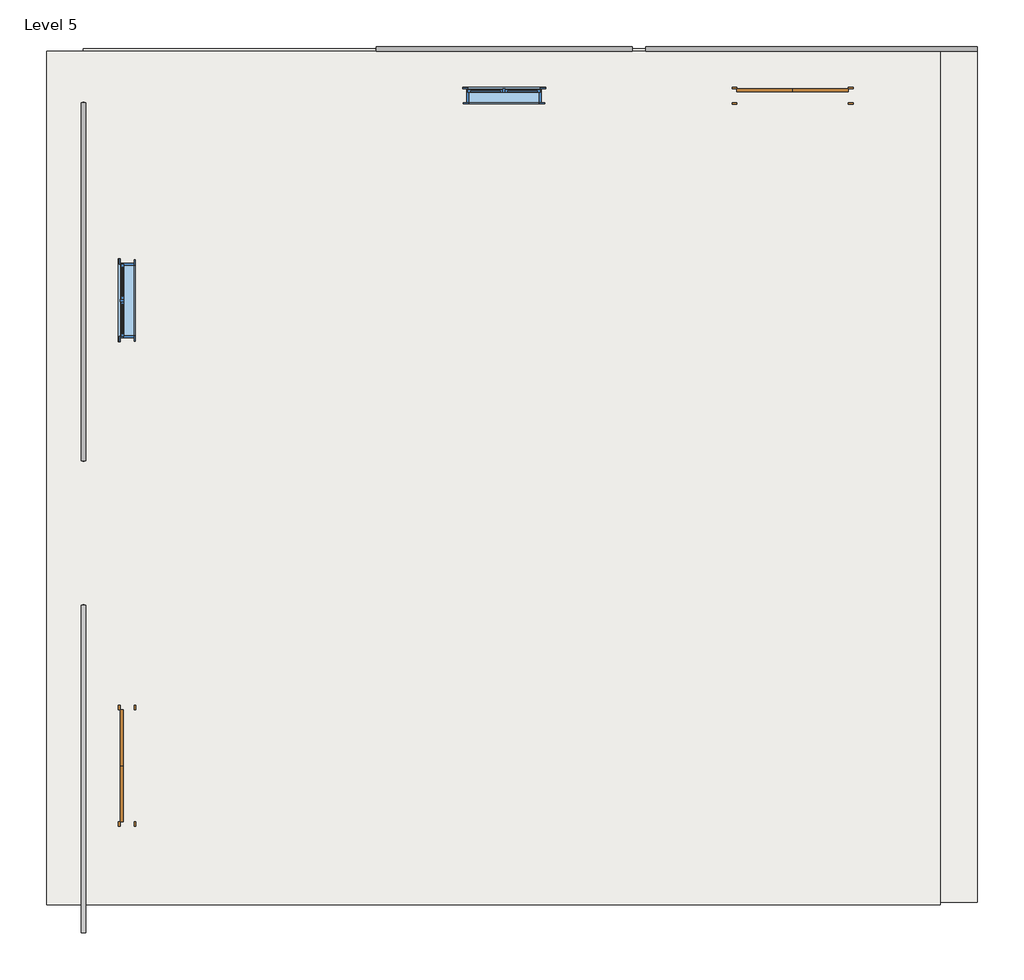
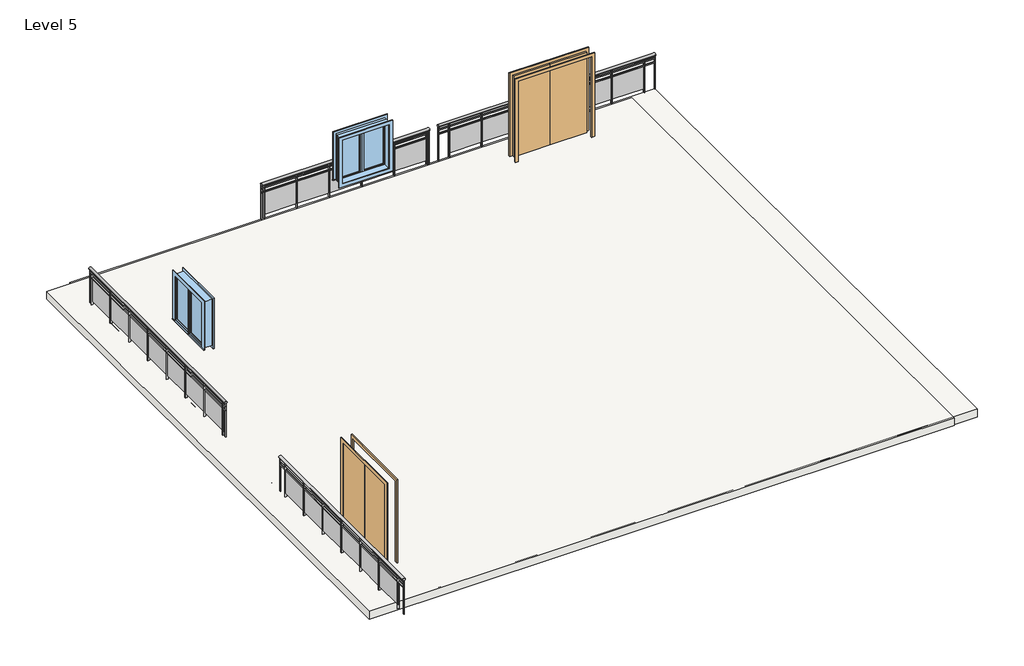
# One storey: 4 railings, 2 doors, 2 slabs, 2 windows.
"""IFC4 building model written with IfcOpenShell, lengths in millimetres."""

from ifc_helpers import new_model, si_unit, point, frame, origin, place, context, project, spatial, polyline, ellipse_curve, trimmed, outline, extrude, transform, mapped, element, save
from ifc_brep_helpers import plane_surface, extruded_surface, advanced_brep
from components import door_640b4634, window_534dcd48

model = new_model("IFC4")

# Units and contexts
model_context = context("Model", 3, world=origin())
ifc_project = project(units=[si_unit("LENGTHUNIT", "METRE", prefix="MILLI")], contexts=[model_context])

# Site, building, storey
site = spatial("IfcSite", under=ifc_project)
building = spatial("IfcBuilding", under=site)
storey = spatial("IfcBuildingStorey", under=building, Name="Level 5", Elevation=12801.6)

# Doors
placement = place(None, origin())
door_shape = door_640b4634(model_context)
element("IfcDoor", 1, ObjectType="Door-Double-Flush_Panel : 72\" x 84\"", at=placement, inside=storey, context=model_context, shape_type="MappedRepresentation", body=[
    mapped(door_shape, transform((-18468.543393, -6784.3397804, 12801.6), x_axis=(0.0, 1.0, 0.0), y_axis=(-1.0, 0.0, 0.0), z_axis=(0.0, 0.0, 1.0))),
])
element("IfcDoor", 2, ObjectType="Door-Double-Flush_Panel : 72\" x 84\"", at=placement, inside=storey, context=model_context, shape_type="MappedRepresentation", body=[
    mapped(door_shape, transform((-7571.943393, 4188.4602196, 12801.6), x_axis=(1.0, 0.0, 0.0), y_axis=(0.0, 1.0, 0.0), z_axis=(0.0, 0.0, 1.0))),
])

# Railings
element("IfcRailing", 3, ObjectType="Glass Panel - Bottom Fill", at=placement, inside=storey, context=model_context, shape_type="SolidModel", body=[
    advanced_brep(
    [(-19220.0296876, -9514.8397804, 13716.0), (-19143.8296876, -9514.8397804, 13716.0), (-19220.0296876, -4155.4397804, 13716.0), (-19143.8296876, -4155.4397804, 13716.0)],
    [
        (0, 1, ellipse_curve(frame((-19181.9296876, -9514.8397804, 13716.0), z_axis=(0.0, -1.0, 0.0), x_axis=(1.0, 0.0, 0.0)), 38.1, 28.575)),
        (1, 0, ellipse_curve(frame((-19181.9296876, -9514.8397804, 13716.0), z_axis=(0.0, -1.0, 0.0), x_axis=(1.0, 0.0, 0.0)), 38.1, 28.575)),
        (2, 3, ellipse_curve(frame((-19181.9296876, -4155.4397804, 13716.0), z_axis=(0.0, 1.0, 0.0), x_axis=(1.0, 0.0, 0.0)), 38.1, 28.575)),
        (3, 2, ellipse_curve(frame((-19181.9296876, -4155.4397804, 13716.0), z_axis=(0.0, 1.0, 0.0), x_axis=(1.0, 0.0, 0.0)), 38.1, 28.575)),
        (0, 2),
        (3, 1),
    ],
    [
        plane_surface(frame((-19181.9296876, -9514.8397804, 13716.0), z_axis=(0.0, -1.0, 0.0), x_axis=(0.0, 0.0, 1.0))),
        plane_surface(frame((-19181.9296876, -4155.4397804, 13716.0), z_axis=(0.0, 1.0, 0.0), x_axis=(0.0, 0.0, 1.0))),
        extruded_surface(trimmed(ellipse_curve(frame((-19181.9296876, -4155.4397804, 13716.0), z_axis=(0.0, -1.0, 0.0), x_axis=(1.0, 0.0, 0.0)), 38.1, 28.575), [point((-19220.0296876, -4155.4397804, 13716.0))], [point((-19143.8296876, -4155.4397804, 13716.0))], True, "CARTESIAN"), (0.0, -5359.4, 0.0), 5359.4),
        extruded_surface(trimmed(ellipse_curve(frame((-19181.9296876, -4155.4397804, 13716.0), z_axis=(0.0, -1.0, 0.0), x_axis=(1.0, 0.0, 0.0)), 38.1, 28.575), [point((-19143.8296876, -4155.4397804, 13716.0))], [point((-19220.0296876, -4155.4397804, 13716.0))], True, "CARTESIAN"), (0.0, -5359.4, 0.0), 5359.4),
    ],
    [
        (0, [[1, 2]]),
        (1, [[3, 4]]),
        (2, [[-1, 5, -4, 6]]),
        (3, [[-2, -6, -3, -5]]),
    ],
),
    extrude(outline(polyline([(-19169.2296876, -9514.8397804), (-19194.6296876, -9514.8397804), (-19194.6296876, -4155.4397804), (-19169.2296876, -4155.4397804), (-19169.2296876, -9514.8397804)])), frame((0.0, 0.0, 13601.7), z_axis=(0.0, 0.0, 1.0), x_axis=(1.0, 0.0, 0.0)), (0.0, 0.0, 1.0), 25.4),
    extrude(outline(polyline([(-19169.2296876, -9514.8397804), (-19194.6296876, -9514.8397804), (-19194.6296876, -4155.4397804), (-19169.2296876, -4155.4397804), (-19169.2296876, -9514.8397804)])), frame((0.0, 0.0, 13500.1), z_axis=(0.0, 0.0, 1.0), x_axis=(1.0, 0.0, 0.0)), (0.0, 0.0, 1.0), 25.4),
    extrude(outline(polyline([(-19156.5296876, -4403.0897804), (-19207.3296876, -4403.0897804), (-19207.3296876, -4390.3897804), (-19156.5296876, -4390.3897804), (-19156.5296876, -4403.0897804)])), frame((0.0, 0.0, 12801.6), z_axis=(0.0, 0.0, 1.0), x_axis=(1.0, 0.0, 0.0)), (0.0, 0.0, 1.0), 885.6788223),
    extrude(outline(polyline([(-19188.4648446, -5209.5397804), (-19188.4648446, -4396.7397804), (-19182.1148446, -4396.7397804), (-19182.1148446, -5209.5397804), (-19188.4648446, -5209.5397804)])), frame((0.0, 0.0, 12903.2), z_axis=(0.0, 0.0, 1.0), x_axis=(1.0, 0.0, 0.0)), (0.0, 0.0, 1.0), 596.9),
    extrude(outline(polyline([(-19156.5296876, -5215.8897804), (-19207.3296876, -5215.8897804), (-19207.3296876, -5203.1897804), (-19156.5296876, -5203.1897804), (-19156.5296876, -5215.8897804)])), frame((0.0, 0.0, 12801.6), z_axis=(0.0, 0.0, 1.0), x_axis=(1.0, 0.0, 0.0)), (0.0, 0.0, 1.0), 885.6788223),
    extrude(outline(polyline([(-19188.4648446, -6022.3397804), (-19188.4648446, -5209.5397804), (-19182.1148446, -5209.5397804), (-19182.1148446, -6022.3397804), (-19188.4648446, -6022.3397804)])), frame((0.0, 0.0, 12903.2), z_axis=(0.0, 0.0, 1.0), x_axis=(1.0, 0.0, 0.0)), (0.0, 0.0, 1.0), 596.9),
    extrude(outline(polyline([(-19156.5296876, -6028.6897804), (-19207.3296876, -6028.6897804), (-19207.3296876, -6015.9897804), (-19156.5296876, -6015.9897804), (-19156.5296876, -6028.6897804)])), frame((0.0, 0.0, 12801.6), z_axis=(0.0, 0.0, 1.0), x_axis=(1.0, 0.0, 0.0)), (0.0, 0.0, 1.0), 885.6788223),
    extrude(outline(polyline([(-19188.4648446, -6835.1397804), (-19188.4648446, -6022.3397804), (-19182.1148446, -6022.3397804), (-19182.1148446, -6835.1397804), (-19188.4648446, -6835.1397804)])), frame((0.0, 0.0, 12903.2), z_axis=(0.0, 0.0, 1.0), x_axis=(1.0, 0.0, 0.0)), (0.0, 0.0, 1.0), 596.9),
    extrude(outline(polyline([(-19156.5296876, -6841.4897804), (-19207.3296876, -6841.4897804), (-19207.3296876, -6828.7897804), (-19156.5296876, -6828.7897804), (-19156.5296876, -6841.4897804)])), frame((0.0, 0.0, 12801.6), z_axis=(0.0, 0.0, 1.0), x_axis=(1.0, 0.0, 0.0)), (0.0, 0.0, 1.0), 885.6788223),
    extrude(outline(polyline([(-19188.4648446, -7647.9397804), (-19188.4648446, -6835.1397804), (-19182.1148446, -6835.1397804), (-19182.1148446, -7647.9397804), (-19188.4648446, -7647.9397804)])), frame((0.0, 0.0, 12903.2), z_axis=(0.0, 0.0, 1.0), x_axis=(1.0, 0.0, 0.0)), (0.0, 0.0, 1.0), 596.9),
    extrude(outline(polyline([(-19156.5296876, -7654.2897804), (-19207.3296876, -7654.2897804), (-19207.3296876, -7641.5897804), (-19156.5296876, -7641.5897804), (-19156.5296876, -7654.2897804)])), frame((0.0, 0.0, 12801.6), z_axis=(0.0, 0.0, 1.0), x_axis=(1.0, 0.0, 0.0)), (0.0, 0.0, 1.0), 885.6788223),
    extrude(outline(polyline([(-19188.4648446, -8460.7397804), (-19188.4648446, -7647.9397804), (-19182.1148446, -7647.9397804), (-19182.1148446, -8460.7397804), (-19188.4648446, -8460.7397804)])), frame((0.0, 0.0, 12903.2), z_axis=(0.0, 0.0, 1.0), x_axis=(1.0, 0.0, 0.0)), (0.0, 0.0, 1.0), 596.9),
    extrude(outline(polyline([(-19156.5296876, -8467.0897804), (-19207.3296876, -8467.0897804), (-19207.3296876, -8454.3897804), (-19156.5296876, -8454.3897804), (-19156.5296876, -8467.0897804)])), frame((0.0, 0.0, 12801.6), z_axis=(0.0, 0.0, 1.0), x_axis=(1.0, 0.0, 0.0)), (0.0, 0.0, 1.0), 885.6788223),
    extrude(outline(polyline([(-19188.4648446, -9273.5397804), (-19188.4648446, -8460.7397804), (-19182.1148446, -8460.7397804), (-19182.1148446, -9273.5397804), (-19188.4648446, -9273.5397804)])), frame((0.0, 0.0, 12903.2), z_axis=(0.0, 0.0, 1.0), x_axis=(1.0, 0.0, 0.0)), (0.0, 0.0, 1.0), 596.9),
    extrude(outline(polyline([(-19156.5296876, -9279.8897804), (-19207.3296876, -9279.8897804), (-19207.3296876, -9267.1897804), (-19156.5296876, -9267.1897804), (-19156.5296876, -9279.8897804)])), frame((0.0, 0.0, 12801.6), z_axis=(0.0, 0.0, 1.0), x_axis=(1.0, 0.0, 0.0)), (0.0, 0.0, 1.0), 885.6788223),
    extrude(outline(polyline([(-19172.4046876, -4168.1397804), (-19191.4546876, -4168.1397804), (-19191.4546876, -4149.0897804), (-19172.4046876, -4149.0897804), (-19172.4046876, -4168.1397804)])), frame((0.0, 0.0, 12801.6), z_axis=(0.0, 0.0, 1.0), x_axis=(1.0, 0.0, 0.0)), (0.0, 0.0, 1.0), 885.6788223),
    extrude(outline(polyline([(-19172.4046876, -9521.1897804), (-19191.4546876, -9521.1897804), (-19191.4546876, -9502.1397804), (-19172.4046876, -9502.1397804), (-19172.4046876, -9521.1897804)])), frame((0.0, 0.0, 12801.6), z_axis=(0.0, 0.0, 1.0), x_axis=(1.0, 0.0, 0.0)), (0.0, 0.0, 1.0), 885.6788223),
])
element("IfcRailing", 4, ObjectType="Glass Panel - Bottom Fill", at=placement, inside=storey, context=model_context, shape_type="SolidModel", body=[
    advanced_brep(
    [(-19143.8296876, 4074.1602196, 13716.0), (-19220.0296876, 4074.1602196, 13716.0), (-19143.8296876, -1793.2397804, 13716.0), (-19220.0296876, -1793.2397804, 13716.0)],
    [
        (0, 1, ellipse_curve(frame((-19181.9296876, 4074.1602196, 13716.0), z_axis=(0.0, 1.0, 0.0), x_axis=(-1.0, 0.0, 0.0)), 38.1, 28.575)),
        (1, 0, ellipse_curve(frame((-19181.9296876, 4074.1602196, 13716.0), z_axis=(0.0, 1.0, 0.0), x_axis=(-1.0, 0.0, 0.0)), 38.1, 28.575)),
        (2, 3, ellipse_curve(frame((-19181.9296876, -1793.2397804, 13716.0), z_axis=(0.0, -1.0, 0.0), x_axis=(-1.0, 0.0, 0.0)), 38.1, 28.575)),
        (3, 2, ellipse_curve(frame((-19181.9296876, -1793.2397804, 13716.0), z_axis=(0.0, -1.0, 0.0), x_axis=(-1.0, 0.0, 0.0)), 38.1, 28.575)),
        (0, 2),
        (3, 1),
    ],
    [
        plane_surface(frame((-19181.9296876, 4074.1602196, 13716.0), z_axis=(0.0, 1.0, 0.0), x_axis=(0.0, 0.0, -1.0))),
        plane_surface(frame((-19181.9296876, -1793.2397804, 13716.0), z_axis=(0.0, -1.0, 0.0), x_axis=(0.0, 0.0, -1.0))),
        extruded_surface(trimmed(ellipse_curve(frame((-19181.9296876, -1793.2397804, 13716.0), z_axis=(0.0, 1.0, 0.0), x_axis=(-1.0, 0.0, 0.0)), 38.1, 28.575), [point((-19143.8296876, -1793.2397804, 13716.0))], [point((-19220.0296876, -1793.2397804, 13716.0))], True, "CARTESIAN"), (0.0, 5867.4, 0.0), 5867.4),
        extruded_surface(trimmed(ellipse_curve(frame((-19181.9296876, -1793.2397804, 13716.0), z_axis=(0.0, 1.0, 0.0), x_axis=(-1.0, 0.0, 0.0)), 38.1, 28.575), [point((-19220.0296876, -1793.2397804, 13716.0))], [point((-19143.8296876, -1793.2397804, 13716.0))], True, "CARTESIAN"), (0.0, 5867.4, 0.0), 5867.4),
    ],
    [
        (0, [[1, 2]]),
        (1, [[3, 4]]),
        (2, [[-1, 5, -4, 6]]),
        (3, [[-2, -6, -3, -5]]),
    ],
),
    extrude(outline(polyline([(-19194.6296876, 4074.1602196), (-19169.2296876, 4074.1602196), (-19169.2296876, -1793.2397804), (-19194.6296876, -1793.2397804), (-19194.6296876, 4074.1602196)])), frame((0.0, 0.0, 13601.7), z_axis=(0.0, 0.0, 1.0), x_axis=(1.0, 0.0, 0.0)), (0.0, 0.0, 1.0), 25.4),
    extrude(outline(polyline([(-19194.6296876, 4074.1602196), (-19169.2296876, 4074.1602196), (-19169.2296876, -1793.2397804), (-19194.6296876, -1793.2397804), (-19194.6296876, 4074.1602196)])), frame((0.0, 0.0, 13500.1), z_axis=(0.0, 0.0, 1.0), x_axis=(1.0, 0.0, 0.0)), (0.0, 0.0, 1.0), 25.4),
    extrude(outline(polyline([(-19207.3296876, -1697.9897804), (-19156.5296876, -1697.9897804), (-19156.5296876, -1710.6897804), (-19207.3296876, -1710.6897804), (-19207.3296876, -1697.9897804)])), frame((0.0, 0.0, 12801.6), z_axis=(0.0, 0.0, 1.0), x_axis=(1.0, 0.0, 0.0)), (0.0, 0.0, 1.0), 885.6788223),
    extrude(outline(polyline([(-19175.3945306, -891.5397804), (-19175.3945306, -1704.3397804), (-19181.7445306, -1704.3397804), (-19181.7445306, -891.5397804), (-19175.3945306, -891.5397804)])), frame((0.0, 0.0, 12903.2), z_axis=(0.0, 0.0, 1.0), x_axis=(1.0, 0.0, 0.0)), (0.0, 0.0, 1.0), 596.9),
    extrude(outline(polyline([(-19207.3296876, -885.1897804), (-19156.5296876, -885.1897804), (-19156.5296876, -897.8897804), (-19207.3296876, -897.8897804), (-19207.3296876, -885.1897804)])), frame((0.0, 0.0, 12801.6), z_axis=(0.0, 0.0, 1.0), x_axis=(1.0, 0.0, 0.0)), (0.0, 0.0, 1.0), 885.6788223),
    extrude(outline(polyline([(-19175.3945306, -78.7397804), (-19175.3945306, -891.5397804), (-19181.7445306, -891.5397804), (-19181.7445306, -78.7397804), (-19175.3945306, -78.7397804)])), frame((0.0, 0.0, 12903.2), z_axis=(0.0, 0.0, 1.0), x_axis=(1.0, 0.0, 0.0)), (0.0, 0.0, 1.0), 596.9),
    extrude(outline(polyline([(-19207.3296876, -72.3897804), (-19156.5296876, -72.3897804), (-19156.5296876, -85.0897804), (-19207.3296876, -85.0897804), (-19207.3296876, -72.3897804)])), frame((0.0, 0.0, 12801.6), z_axis=(0.0, 0.0, 1.0), x_axis=(1.0, 0.0, 0.0)), (0.0, 0.0, 1.0), 885.6788223),
    extrude(outline(polyline([(-19175.3945306, 734.0602196), (-19175.3945306, -78.7397804), (-19181.7445306, -78.7397804), (-19181.7445306, 734.0602196), (-19175.3945306, 734.0602196)])), frame((0.0, 0.0, 12903.2), z_axis=(0.0, 0.0, 1.0), x_axis=(1.0, 0.0, 0.0)), (0.0, 0.0, 1.0), 596.9),
    extrude(outline(polyline([(-19207.3296876, 740.4102196), (-19156.5296876, 740.4102196), (-19156.5296876, 727.7102196), (-19207.3296876, 727.7102196), (-19207.3296876, 740.4102196)])), frame((0.0, 0.0, 12801.6), z_axis=(0.0, 0.0, 1.0), x_axis=(1.0, 0.0, 0.0)), (0.0, 0.0, 1.0), 885.6788223),
    extrude(outline(polyline([(-19175.3945306, 1546.8602196), (-19175.3945306, 734.0602196), (-19181.7445306, 734.0602196), (-19181.7445306, 1546.8602196), (-19175.3945306, 1546.8602196)])), frame((0.0, 0.0, 12903.2), z_axis=(0.0, 0.0, 1.0), x_axis=(1.0, 0.0, 0.0)), (0.0, 0.0, 1.0), 596.9),
    extrude(outline(polyline([(-19207.3296876, 1553.2102196), (-19156.5296876, 1553.2102196), (-19156.5296876, 1540.5102196), (-19207.3296876, 1540.5102196), (-19207.3296876, 1553.2102196)])), frame((0.0, 0.0, 12801.6), z_axis=(0.0, 0.0, 1.0), x_axis=(1.0, 0.0, 0.0)), (0.0, 0.0, 1.0), 885.6788223),
    extrude(outline(polyline([(-19175.3945306, 2359.6602196), (-19175.3945306, 1546.8602196), (-19181.7445306, 1546.8602196), (-19181.7445306, 2359.6602196), (-19175.3945306, 2359.6602196)])), frame((0.0, 0.0, 12903.2), z_axis=(0.0, 0.0, 1.0), x_axis=(1.0, 0.0, 0.0)), (0.0, 0.0, 1.0), 596.9),
    extrude(outline(polyline([(-19207.3296876, 2366.0102196), (-19156.5296876, 2366.0102196), (-19156.5296876, 2353.3102196), (-19207.3296876, 2353.3102196), (-19207.3296876, 2366.0102196)])), frame((0.0, 0.0, 12801.6), z_axis=(0.0, 0.0, 1.0), x_axis=(1.0, 0.0, 0.0)), (0.0, 0.0, 1.0), 885.6788223),
    extrude(outline(polyline([(-19175.3945306, 3172.4602196), (-19175.3945306, 2359.6602196), (-19181.7445306, 2359.6602196), (-19181.7445306, 3172.4602196), (-19175.3945306, 3172.4602196)])), frame((0.0, 0.0, 12903.2), z_axis=(0.0, 0.0, 1.0), x_axis=(1.0, 0.0, 0.0)), (0.0, 0.0, 1.0), 596.9),
    extrude(outline(polyline([(-19207.3296876, 3178.8102196), (-19156.5296876, 3178.8102196), (-19156.5296876, 3166.1102196), (-19207.3296876, 3166.1102196), (-19207.3296876, 3178.8102196)])), frame((0.0, 0.0, 12801.6), z_axis=(0.0, 0.0, 1.0), x_axis=(1.0, 0.0, 0.0)), (0.0, 0.0, 1.0), 885.6788223),
    extrude(outline(polyline([(-19175.3945306, 3985.2602196), (-19175.3945306, 3172.4602196), (-19181.7445306, 3172.4602196), (-19181.7445306, 3985.2602196), (-19175.3945306, 3985.2602196)])), frame((0.0, 0.0, 12903.2), z_axis=(0.0, 0.0, 1.0), x_axis=(1.0, 0.0, 0.0)), (0.0, 0.0, 1.0), 596.9),
    extrude(outline(polyline([(-19207.3296876, 3991.6102196), (-19156.5296876, 3991.6102196), (-19156.5296876, 3978.9102196), (-19207.3296876, 3978.9102196), (-19207.3296876, 3991.6102196)])), frame((0.0, 0.0, 12801.6), z_axis=(0.0, 0.0, 1.0), x_axis=(1.0, 0.0, 0.0)), (0.0, 0.0, 1.0), 885.6788223),
    extrude(outline(polyline([(-19191.4546876, -1780.5397804), (-19172.4046876, -1780.5397804), (-19172.4046876, -1799.5897804), (-19191.4546876, -1799.5897804), (-19191.4546876, -1780.5397804)])), frame((0.0, 0.0, 12801.6), z_axis=(0.0, 0.0, 1.0), x_axis=(1.0, 0.0, 0.0)), (0.0, 0.0, 1.0), 885.6788223),
    extrude(outline(polyline([(-19191.4546876, 4080.5102196), (-19172.4046876, 4080.5102196), (-19172.4046876, 4061.4602196), (-19191.4546876, 4061.4602196), (-19191.4546876, 4080.5102196)])), frame((0.0, 0.0, 12801.6), z_axis=(0.0, 0.0, 1.0), x_axis=(1.0, 0.0, 0.0)), (0.0, 0.0, 1.0), 885.6788223),
])
element("IfcRailing", 5, ObjectType="Glass Panel - Bottom Fill", at=placement, inside=storey, context=model_context, shape_type="SolidModel", body=[
    advanced_brep(
    [(-14391.843393, 4991.4940048, 13716.0), (-14391.843393, 4915.2940048, 13716.0), (-10200.843393, 4991.4940048, 13716.0), (-10200.843393, 4915.2940048, 13716.0)],
    [
        (0, 1, ellipse_curve(frame((-14391.843393, 4953.3940048, 13716.0), z_axis=(-1.0, 0.0, 0.0), x_axis=(0.0, -1.0, 0.0)), 38.1, 28.575)),
        (1, 0, ellipse_curve(frame((-14391.843393, 4953.3940048, 13716.0), z_axis=(-1.0, 0.0, 0.0), x_axis=(0.0, -1.0, 0.0)), 38.1, 28.575)),
        (2, 3, ellipse_curve(frame((-10200.843393, 4953.3940048, 13716.0), z_axis=(1.0, 0.0, 0.0), x_axis=(0.0, -1.0, 0.0)), 38.1, 28.575)),
        (3, 2, ellipse_curve(frame((-10200.843393, 4953.3940048, 13716.0), z_axis=(1.0, 0.0, 0.0), x_axis=(0.0, -1.0, 0.0)), 38.1, 28.575)),
        (0, 2),
        (3, 1),
    ],
    [
        plane_surface(frame((-14391.843393, 4953.3940048, 13716.0), z_axis=(-1.0, 0.0, 0.0), x_axis=(0.0, 1.0, 0.0))),
        plane_surface(frame((-10200.843393, 4953.3940048, 13716.0), z_axis=(1.0, 0.0, 0.0), x_axis=(0.0, 1.0, 0.0))),
        extruded_surface(trimmed(ellipse_curve(frame((-10200.843393, 4953.3940048, 13716.0), z_axis=(-1.0, 0.0, 0.0), x_axis=(0.0, -1.0, 0.0)), 38.1, 28.575), [point((-10200.843393, 4991.4940048, 13716.0))], [point((-10200.843393, 4915.2940048, 13716.0))], True, "CARTESIAN"), (-4191.0, 0.0, 0.0), 4191.0),
        extruded_surface(trimmed(ellipse_curve(frame((-10200.843393, 4953.3940048, 13716.0), z_axis=(-1.0, 0.0, 0.0), x_axis=(0.0, -1.0, 0.0)), 38.1, 28.575), [point((-10200.843393, 4915.2940048, 13716.0))], [point((-10200.843393, 4991.4940048, 13716.0))], True, "CARTESIAN"), (-4191.0, 0.0, 0.0), 4191.0),
    ],
    [
        (0, [[1, 2]]),
        (1, [[3, 4]]),
        (2, [[-1, 5, -4, 6]]),
        (3, [[-2, -6, -3, -5]]),
    ],
),
    extrude(outline(polyline([(-14391.843393, 4940.6940048), (-14391.843393, 4966.0940048), (-10200.843393, 4966.0940048), (-10200.843393, 4940.6940048), (-14391.843393, 4940.6940048)])), frame((0.0, 0.0, 13601.7), z_axis=(0.0, 0.0, 1.0), x_axis=(1.0, 0.0, 0.0)), (0.0, 0.0, 1.0), 25.4),
    extrude(outline(polyline([(-14391.843393, 4940.6940048), (-14391.843393, 4966.0940048), (-10200.843393, 4966.0940048), (-10200.843393, 4940.6940048), (-14391.843393, 4940.6940048)])), frame((0.0, 0.0, 13500.1), z_axis=(0.0, 0.0, 1.0), x_axis=(1.0, 0.0, 0.0)), (0.0, 0.0, 1.0), 25.4),
    extrude(outline(polyline([(-10270.693393, 4927.9940048), (-10270.693393, 4978.7940048), (-10257.993393, 4978.7940048), (-10257.993393, 4927.9940048), (-10270.693393, 4927.9940048)])), frame((0.0, 0.0, 12801.6), z_axis=(0.0, 0.0, 1.0), x_axis=(1.0, 0.0, 0.0)), (0.0, 0.0, 1.0), 885.6788223),
    extrude(outline(polyline([(-11077.143393, 4959.9291618), (-10264.343393, 4959.9291618), (-10264.343393, 4953.5791618), (-11077.143393, 4953.5791618), (-11077.143393, 4959.9291618)])), frame((0.0, 0.0, 12903.2), z_axis=(0.0, 0.0, 1.0), x_axis=(1.0, 0.0, 0.0)), (0.0, 0.0, 1.0), 596.9),
    extrude(outline(polyline([(-11083.493393, 4927.9940048), (-11083.493393, 4978.7940048), (-11070.793393, 4978.7940048), (-11070.793393, 4927.9940048), (-11083.493393, 4927.9940048)])), frame((0.0, 0.0, 12801.6), z_axis=(0.0, 0.0, 1.0), x_axis=(1.0, 0.0, 0.0)), (0.0, 0.0, 1.0), 885.6788223),
    extrude(outline(polyline([(-11889.943393, 4959.9291618), (-11077.143393, 4959.9291618), (-11077.143393, 4953.5791618), (-11889.943393, 4953.5791618), (-11889.943393, 4959.9291618)])), frame((0.0, 0.0, 12903.2), z_axis=(0.0, 0.0, 1.0), x_axis=(1.0, 0.0, 0.0)), (0.0, 0.0, 1.0), 596.9),
    extrude(outline(polyline([(-11896.293393, 4927.9940048), (-11896.293393, 4978.7940048), (-11883.593393, 4978.7940048), (-11883.593393, 4927.9940048), (-11896.293393, 4927.9940048)])), frame((0.0, 0.0, 12801.6), z_axis=(0.0, 0.0, 1.0), x_axis=(1.0, 0.0, 0.0)), (0.0, 0.0, 1.0), 885.6788223),
    extrude(outline(polyline([(-12702.743393, 4959.9291618), (-11889.943393, 4959.9291618), (-11889.943393, 4953.5791618), (-12702.743393, 4953.5791618), (-12702.743393, 4959.9291618)])), frame((0.0, 0.0, 12903.2), z_axis=(0.0, 0.0, 1.0), x_axis=(1.0, 0.0, 0.0)), (0.0, 0.0, 1.0), 596.9),
    extrude(outline(polyline([(-12709.093393, 4927.9940048), (-12709.093393, 4978.7940048), (-12696.393393, 4978.7940048), (-12696.393393, 4927.9940048), (-12709.093393, 4927.9940048)])), frame((0.0, 0.0, 12801.6), z_axis=(0.0, 0.0, 1.0), x_axis=(1.0, 0.0, 0.0)), (0.0, 0.0, 1.0), 885.6788223),
    extrude(outline(polyline([(-13515.543393, 4959.9291618), (-12702.743393, 4959.9291618), (-12702.743393, 4953.5791618), (-13515.543393, 4953.5791618), (-13515.543393, 4959.9291618)])), frame((0.0, 0.0, 12903.2), z_axis=(0.0, 0.0, 1.0), x_axis=(1.0, 0.0, 0.0)), (0.0, 0.0, 1.0), 596.9),
    extrude(outline(polyline([(-13521.893393, 4927.9940048), (-13521.893393, 4978.7940048), (-13509.193393, 4978.7940048), (-13509.193393, 4927.9940048), (-13521.893393, 4927.9940048)])), frame((0.0, 0.0, 12801.6), z_axis=(0.0, 0.0, 1.0), x_axis=(1.0, 0.0, 0.0)), (0.0, 0.0, 1.0), 885.6788223),
    extrude(outline(polyline([(-14328.343393, 4959.9291618), (-13515.543393, 4959.9291618), (-13515.543393, 4953.5791618), (-14328.343393, 4953.5791618), (-14328.343393, 4959.9291618)])), frame((0.0, 0.0, 12903.2), z_axis=(0.0, 0.0, 1.0), x_axis=(1.0, 0.0, 0.0)), (0.0, 0.0, 1.0), 596.9),
    extrude(outline(polyline([(-14334.693393, 4927.9940048), (-14334.693393, 4978.7940048), (-14321.993393, 4978.7940048), (-14321.993393, 4927.9940048), (-14334.693393, 4927.9940048)])), frame((0.0, 0.0, 12801.6), z_axis=(0.0, 0.0, 1.0), x_axis=(1.0, 0.0, 0.0)), (0.0, 0.0, 1.0), 885.6788223),
    extrude(outline(polyline([(-10213.543393, 4943.8690048), (-10213.543393, 4962.9190048), (-10194.493393, 4962.9190048), (-10194.493393, 4943.8690048), (-10213.543393, 4943.8690048)])), frame((0.0, 0.0, 12801.6), z_axis=(0.0, 0.0, 1.0), x_axis=(1.0, 0.0, 0.0)), (0.0, 0.0, 1.0), 885.6788223),
    extrude(outline(polyline([(-14398.193393, 4943.8690048), (-14398.193393, 4962.9190048), (-14379.143393, 4962.9190048), (-14379.143393, 4943.8690048), (-14398.193393, 4943.8690048)])), frame((0.0, 0.0, 12801.6), z_axis=(0.0, 0.0, 1.0), x_axis=(1.0, 0.0, 0.0)), (0.0, 0.0, 1.0), 885.6788223),
])
element("IfcRailing", 6, ObjectType="Glass Panel - Bottom Fill", at=placement, inside=storey, context=model_context, shape_type="SolidModel", body=[
    advanced_brep(
    [(-9972.243393, 4991.4940048, 13716.0), (-9972.243393, 4915.2940048, 13716.0), (-4551.5296876, 4991.4940048, 13716.0), (-4551.5296876, 4915.2940048, 13716.0)],
    [
        (0, 1, ellipse_curve(frame((-9972.243393, 4953.3940048, 13716.0), z_axis=(-1.0, 0.0, 0.0), x_axis=(0.0, -1.0, 0.0)), 38.1, 28.575)),
        (1, 0, ellipse_curve(frame((-9972.243393, 4953.3940048, 13716.0), z_axis=(-1.0, 0.0, 0.0), x_axis=(0.0, -1.0, 0.0)), 38.1, 28.575)),
        (2, 3, ellipse_curve(frame((-4551.5296876, 4953.3940048, 13716.0), z_axis=(1.0, 0.0, 0.0), x_axis=(0.0, -1.0, 0.0)), 38.1, 28.575)),
        (3, 2, ellipse_curve(frame((-4551.5296876, 4953.3940048, 13716.0), z_axis=(1.0, 0.0, 0.0), x_axis=(0.0, -1.0, 0.0)), 38.1, 28.575)),
        (0, 2),
        (3, 1),
    ],
    [
        plane_surface(frame((-9972.243393, 4953.3940048, 13716.0), z_axis=(-1.0, 0.0, 0.0), x_axis=(0.0, 1.0, 0.0))),
        plane_surface(frame((-4551.5296876, 4953.3940048, 13716.0), z_axis=(1.0, 0.0, 0.0), x_axis=(0.0, 1.0, 0.0))),
        extruded_surface(trimmed(ellipse_curve(frame((-4551.5296876, 4953.3940048, 13716.0), z_axis=(-1.0, 0.0, 0.0), x_axis=(0.0, -1.0, 0.0)), 38.1, 28.575), [point((-4551.5296876, 4991.4940048, 13716.0))], [point((-4551.5296876, 4915.2940048, 13716.0))], True, "CARTESIAN"), (-5420.7137054, 0.0, 0.0), 5420.7137054),
        extruded_surface(trimmed(ellipse_curve(frame((-4551.5296876, 4953.3940048, 13716.0), z_axis=(-1.0, 0.0, 0.0), x_axis=(0.0, -1.0, 0.0)), 38.1, 28.575), [point((-4551.5296876, 4915.2940048, 13716.0))], [point((-4551.5296876, 4991.4940048, 13716.0))], True, "CARTESIAN"), (-5420.7137054, 0.0, 0.0), 5420.7137054),
    ],
    [
        (0, [[1, 2]]),
        (1, [[3, 4]]),
        (2, [[-1, 5, -4, 6]]),
        (3, [[-2, -6, -3, -5]]),
    ],
),
    extrude(outline(polyline([(-9972.243393, 4940.6940048), (-9972.243393, 4966.0940048), (-4551.5296876, 4966.0940048), (-4551.5296876, 4940.6940048), (-9972.243393, 4940.6940048)])), frame((0.0, 0.0, 13601.7), z_axis=(0.0, 0.0, 1.0), x_axis=(1.0, 0.0, 0.0)), (0.0, 0.0, 1.0), 25.4),
    extrude(outline(polyline([(-9972.243393, 4940.6940048), (-9972.243393, 4966.0940048), (-4551.5296876, 4966.0940048), (-4551.5296876, 4940.6940048), (-9972.243393, 4940.6940048)])), frame((0.0, 0.0, 13500.1), z_axis=(0.0, 0.0, 1.0), x_axis=(1.0, 0.0, 0.0)), (0.0, 0.0, 1.0), 25.4),
    extrude(outline(polyline([(-4829.8365403, 4927.9940048), (-4829.8365403, 4978.7940048), (-4817.1365403, 4978.7940048), (-4817.1365403, 4927.9940048), (-4829.8365403, 4927.9940048)])), frame((0.0, 0.0, 12801.6), z_axis=(0.0, 0.0, 1.0), x_axis=(1.0, 0.0, 0.0)), (0.0, 0.0, 1.0), 885.6788223),
    extrude(outline(polyline([(-5636.2865403, 4959.9291618), (-4823.4865403, 4959.9291618), (-4823.4865403, 4953.5791618), (-5636.2865403, 4953.5791618), (-5636.2865403, 4959.9291618)])), frame((0.0, 0.0, 12903.2), z_axis=(0.0, 0.0, 1.0), x_axis=(1.0, 0.0, 0.0)), (0.0, 0.0, 1.0), 596.9),
    extrude(outline(polyline([(-5642.6365403, 4927.9940048), (-5642.6365403, 4978.7940048), (-5629.9365403, 4978.7940048), (-5629.9365403, 4927.9940048), (-5642.6365403, 4927.9940048)])), frame((0.0, 0.0, 12801.6), z_axis=(0.0, 0.0, 1.0), x_axis=(1.0, 0.0, 0.0)), (0.0, 0.0, 1.0), 885.6788223),
    extrude(outline(polyline([(-6449.0865403, 4959.9291618), (-5636.2865403, 4959.9291618), (-5636.2865403, 4953.5791618), (-6449.0865403, 4953.5791618), (-6449.0865403, 4959.9291618)])), frame((0.0, 0.0, 12903.2), z_axis=(0.0, 0.0, 1.0), x_axis=(1.0, 0.0, 0.0)), (0.0, 0.0, 1.0), 596.9),
    extrude(outline(polyline([(-6455.4365403, 4927.9940048), (-6455.4365403, 4978.7940048), (-6442.7365403, 4978.7940048), (-6442.7365403, 4927.9940048), (-6455.4365403, 4927.9940048)])), frame((0.0, 0.0, 12801.6), z_axis=(0.0, 0.0, 1.0), x_axis=(1.0, 0.0, 0.0)), (0.0, 0.0, 1.0), 885.6788223),
    extrude(outline(polyline([(-7261.8865403, 4959.9291618), (-6449.0865403, 4959.9291618), (-6449.0865403, 4953.5791618), (-7261.8865403, 4953.5791618), (-7261.8865403, 4959.9291618)])), frame((0.0, 0.0, 12903.2), z_axis=(0.0, 0.0, 1.0), x_axis=(1.0, 0.0, 0.0)), (0.0, 0.0, 1.0), 596.9),
    extrude(outline(polyline([(-7268.2365403, 4927.9940048), (-7268.2365403, 4978.7940048), (-7255.5365403, 4978.7940048), (-7255.5365403, 4927.9940048), (-7268.2365403, 4927.9940048)])), frame((0.0, 0.0, 12801.6), z_axis=(0.0, 0.0, 1.0), x_axis=(1.0, 0.0, 0.0)), (0.0, 0.0, 1.0), 885.6788223),
    extrude(outline(polyline([(-8074.6865403, 4959.9291618), (-7261.8865403, 4959.9291618), (-7261.8865403, 4953.5791618), (-8074.6865403, 4953.5791618), (-8074.6865403, 4959.9291618)])), frame((0.0, 0.0, 12903.2), z_axis=(0.0, 0.0, 1.0), x_axis=(1.0, 0.0, 0.0)), (0.0, 0.0, 1.0), 596.9),
    extrude(outline(polyline([(-8081.0365403, 4927.9940048), (-8081.0365403, 4978.7940048), (-8068.3365403, 4978.7940048), (-8068.3365403, 4927.9940048), (-8081.0365403, 4927.9940048)])), frame((0.0, 0.0, 12801.6), z_axis=(0.0, 0.0, 1.0), x_axis=(1.0, 0.0, 0.0)), (0.0, 0.0, 1.0), 885.6788223),
    extrude(outline(polyline([(-8887.4865403, 4959.9291618), (-8074.6865403, 4959.9291618), (-8074.6865403, 4953.5791618), (-8887.4865403, 4953.5791618), (-8887.4865403, 4959.9291618)])), frame((0.0, 0.0, 12903.2), z_axis=(0.0, 0.0, 1.0), x_axis=(1.0, 0.0, 0.0)), (0.0, 0.0, 1.0), 596.9),
    extrude(outline(polyline([(-8893.8365403, 4927.9940048), (-8893.8365403, 4978.7940048), (-8881.1365403, 4978.7940048), (-8881.1365403, 4927.9940048), (-8893.8365403, 4927.9940048)])), frame((0.0, 0.0, 12801.6), z_axis=(0.0, 0.0, 1.0), x_axis=(1.0, 0.0, 0.0)), (0.0, 0.0, 1.0), 885.6788223),
    extrude(outline(polyline([(-9700.2865403, 4959.9291618), (-8887.4865403, 4959.9291618), (-8887.4865403, 4953.5791618), (-9700.2865403, 4953.5791618), (-9700.2865403, 4959.9291618)])), frame((0.0, 0.0, 12903.2), z_axis=(0.0, 0.0, 1.0), x_axis=(1.0, 0.0, 0.0)), (0.0, 0.0, 1.0), 596.9),
    extrude(outline(polyline([(-9706.6365403, 4927.9940048), (-9706.6365403, 4978.7940048), (-9693.9365403, 4978.7940048), (-9693.9365403, 4927.9940048), (-9706.6365403, 4927.9940048)])), frame((0.0, 0.0, 12801.6), z_axis=(0.0, 0.0, 1.0), x_axis=(1.0, 0.0, 0.0)), (0.0, 0.0, 1.0), 885.6788223),
    extrude(outline(polyline([(-4564.2296876, 4943.8690048), (-4564.2296876, 4962.9190048), (-4545.1796876, 4962.9190048), (-4545.1796876, 4943.8690048), (-4564.2296876, 4943.8690048)])), frame((0.0, 0.0, 12801.6), z_axis=(0.0, 0.0, 1.0), x_axis=(1.0, 0.0, 0.0)), (0.0, 0.0, 1.0), 885.6788223),
    extrude(outline(polyline([(-9978.593393, 4943.8690048), (-9978.593393, 4962.9190048), (-9959.543393, 4962.9190048), (-9959.543393, 4943.8690048), (-9978.593393, 4943.8690048)])), frame((0.0, 0.0, 12801.6), z_axis=(0.0, 0.0, 1.0), x_axis=(1.0, 0.0, 0.0)), (0.0, 0.0, 1.0), 885.6788223),
])

# Slabs
element("IfcSlab", 7, ObjectType="Generic - 12\"", at=placement, inside=storey, context=model_context, shape_type="SweptSolid", body=[
    extrude(outline(polyline([(-4551.5296876, 4953.3940048), (-4551.5296876, -9017.7838841), (-19181.9296876, -9017.7838841), (-19181.9296876, 4953.3940048), (-4551.5296876, 4953.3940048)])), frame((0.0, 0.0, 12598.4), z_axis=(0.0, 0.0, 1.0), x_axis=(1.0, 0.0, 0.0)), (0.0, 0.0, 1.0), 203.2),
])
element("IfcSlab", 8, ObjectType="Generic - 12\"", at=placement, inside=storey, context=model_context, shape_type="SweptSolid", body=[
    extrude(outline(polyline([(-5155.8153052, 4915.0176665), (-5155.8153052, -9056.1602225), (-19786.2153052, -9056.1602225), (-19786.2153052, 4915.0176665), (-5155.8153052, 4915.0176665)])), frame((0.0, 0.0, 12598.4), z_axis=(0.0, 0.0, 1.0), x_axis=(1.0, 0.0, 0.0)), (0.0, 0.0, 1.0), 203.2),
])

# Windows
window_shape = window_534dcd48(model_context)
element("IfcWindow", 9, ObjectType="Casement Dbl with Trim : 48\" x 48\"", at=placement, inside=storey, context=model_context, shape_type="MappedRepresentation", body=[
    mapped(window_shape, transform((-18449.493393, 835.6602196, 12801.6), x_axis=(0.0, 1.0, 0.0), y_axis=(-1.0, 0.0, 0.0), z_axis=(0.0, 0.0, 1.0))),
])
element("IfcWindow", 10, ObjectType="Casement Dbl with Trim : 48\" x 48\"", at=placement, inside=storey, context=model_context, shape_type="MappedRepresentation", body=[
    mapped(window_shape, transform((-12296.343393, 4169.4102196, 12801.6), x_axis=(1.0, 0.0, 0.0), y_axis=(0.0, 1.0, 0.0), z_axis=(0.0, 0.0, 1.0))),
])

save(model, "model.ifc")

# Revit data of these elements
# Type "Door-Double-Flush_Panel : 72\" x 84\""
#   Type Mark = "11"
#   Construction Type Id = "DOOR"
#   Assembly Code = "C1020"
#   Analytic Construction = "Wooden"
#   Thickness = 0' - 2"
#   Thermal Resistance (R) = 2.5876 (h·ft²·°F)/BTU
#   Swing Angle [instance default] = 90.00°
#   Panel Width = 3' - 0"
#   Heat Transfer Coefficient (U) = 0.3865 BTU/(h·ft²·°F)
#   Height = 7' - 0"
#   Trim Projection Ext = 0' - 1"
#   Trim Projection Int = 0' - 1"
#   Trim Width = 0' - 3"
#   Width = 6' - 0"
#   Define Thermal Properties by = 1
#   Panel Material = Glass, Clear Glazing
#   Trim Material = Paint - Sienna
#   Visual Light Transmittance = 0
#   Solar Heat Gain Coefficient = 0
#   Function = (empty or 0)
#   Wall Closure = (empty or 0)
# Type "Glass Panel - Bottom Fill"
#   Assembly Code = "C2010400"
#   built-in parameter 1008612 = 0.0416667 (stored number, unit not read)
#   built-in parameter 1008611 = 0.0416667 (stored number, unit not read)
#   built-in parameter 1008609 = 0.333333 (stored number, unit not read)
#   built-in parameter 1008604 = 0.166667 (stored number, unit not read)
#   built-in parameter 1008603 = 0.166667 (stored number, unit not read)
#   Railing Height = 3' - 0"
#   built-in parameter 1008630 = 2
#   built-in parameter 1008610 = 2
#   built-in parameter 1008618 = Baluster - Square : 3/4"
# Type "Generic - 12\""
#   Assembly Code = "B1010"
#   Function = 0
#   Layers, outside or top first: 0' - 8" no material (function 1)
# Type "Casement Dbl with Trim : 48\" x 48\""
#   Type Mark = "10"
#   Construction Type Id = "GSP4R"
#   Assembly Code = "B2020100"
#   Analytic Construction = "1/8 in Pilkington single glazing"
#   Visual Light Transmittance = 0.9
#   Solar Heat Gain Coefficient = 0.78
#   Heat Transfer Coefficient (U) = 0.6496 BTU/(h·ft²·°F)
#   Height = 4' - 0"
#   Default Sill Height = 3' - 0"
#   Trim Projection - Ext. = 0' - 0 1/2"
#   Trim Projection - Int. = 0' - 0 3/4"
#   Trim Width - Exterior = 0' - 3 1/2"
#   Trim Width - Interior = 0' - 3 1/2"
#   Width = 4' - 0"
#   Window Inset = 0' - 0 3/4"
#   Define Thermal Properties by = 1
#   Glass Pane Material = Glass
#   Sash Material = Glass, Clear Glazing
#   Trim Exterior Material = Earth
#   Trim Interior Material = Trim
#   Wall Closure = (empty or 0)
# Elements 1, 2 (IfcDoor, "Door-Double-Flush_Panel : 72\" x 84\"")
#   Swing Angle = 90.00°
#   Phase Created = New Construction
#   Materials on its faces: "Paint - Sienna", "Glass, Clear Glazing"
# Elements 3, 4, 5, 6 (IfcRailing, "Glass Panel - Bottom Fill")
#   Phase Created = New Construction
#   Materials on its faces: "Glass"
# Elements 7, 8 (IfcSlab, "Generic - 12\"")
#   Height Offset From Level = 0' - 0"
#   Phase Created = New Construction
#   Materials on its faces: "Default Floor"
# Element 9 (IfcWindow, "Casement Dbl with Trim : 48\" x 48\"")
#   Mark = "4"
#   Phase Created = New Construction
#   Materials on its faces: "Glass, Clear Glazing", "Earth", "Glass", "Trim"
# Element 10 (IfcWindow, "Casement Dbl with Trim : 48\" x 48\"")
#   Mark = "5"
#   Phase Created = New Construction
#   Materials on its faces: "Glass, Clear Glazing", "Earth", "Glass", "Trim"
# Materials
#   "Glass, Clear Glazing": class "Glass", colour RGB 0 128 192, transparency 0.75, Description = "Clear glazing", Cost = 0
#   "Paint - Sienna": colour RGB 118 70 51, transparency 0, Cost = 0
#   "Glass": class "Glass", colour RGB 0 128 192, transparency 0.75, Description = "Soda Lime Glass", Cost = 0
#   "Earth": class "Generic", colour RGB 97 75 62, transparency 0, Description = "Soil", Cost = 0
#   "Trim": class "Wood", colour RGB 224 178 126, transparency 0
#   "Default Floor": colour RGB 128 128 128, transparency 0
